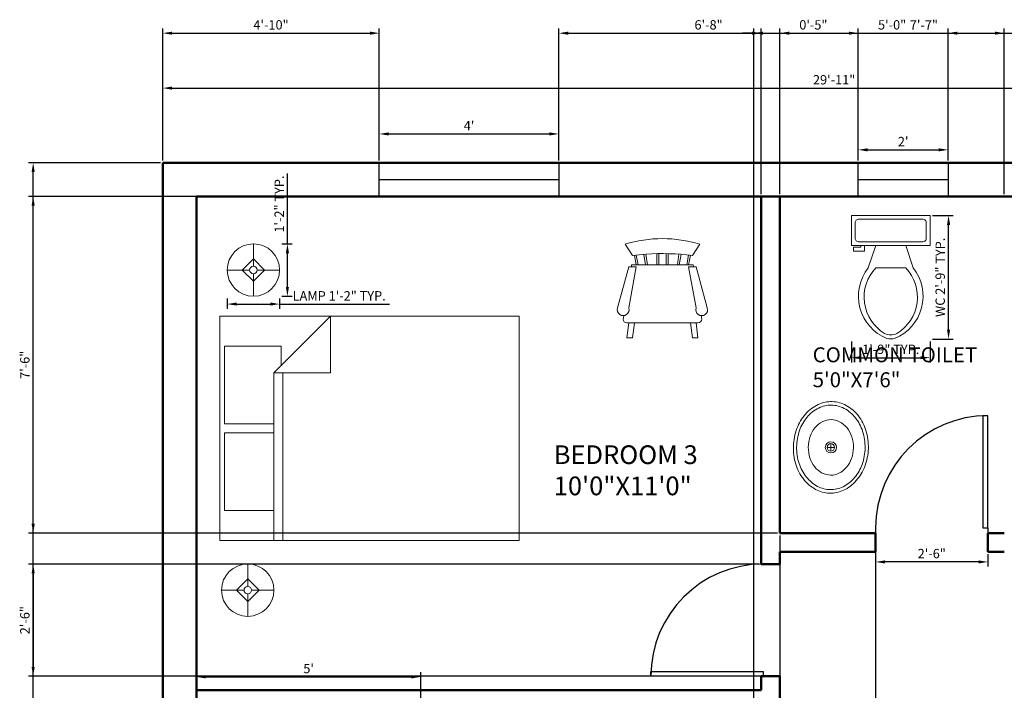
# Model space of a CAD drawing. Units: inches. Extents: x 25547 to 25983, y 30413 to 31159.
# Tile 4 of 5: x 25549 to 25813, y 30978 to 31157. Entities that reach past the tile are written whole.
import ezdxf

# ---------------------------------------------------------------- set-up
doc = ezdxf.new("R2010")
doc.units = ezdxf.units.IN
for name, color, linetype, lineweight in [('A-AREA-IDEN', 11, 'Continuous', 25), ('A-FLOR-FIXT', 6, 'Continuous', 18), ('A-WALL', 7, 'Continuous', 50), ('DIM', 4, 'Continuous', 18), ('DOOR', 3, 'Continuous', 25), ('FURNITURES', 6, 'Continuous', 18), ('WINDOW', 1, 'Continuous', 25)]:
    doc.layers.add(name, color=color, linetype=linetype, lineweight=lineweight)
doc.styles.get("Standard").update_dxf_attribs({"font": 'arial.ttf'})
doc.dimstyles.new('ISO-25', dxfattribs={"dimtxt": 2.5, "dimasz": 2.5, "dimexe": 1.25, "dimexo": 0.625, "dimtad": 1, "dimlunit": 3, "dimtxsty": 'Standard', "dimcen": 2.5, "dimadec": 0, "dimazin": 0, "dimtfac": 1, "dimtmove": 0, "dimatfit": 3, "dimfxl": 1, "dimarcsym": 0})

# ---------------------------------------------------------------- blocks, each defined once
blk = doc.blocks.new('*U5')
for p, q in [((0, 0), (0, -6)), ((40, 0), (40, -6))]:
    blk.add_line(p, q)
blk.add_lwpolyline([(0, 0), (0, 40), (1.75, 40), (1.75, 0)], close=True)
blk.add_arc((0, 0), 40, 0, 90)
blk = doc.blocks.new('*U3')
for p, q in [((0, 0), (0, -6)), ((-40, 0), (-40, -6))]:
    blk.add_line(p, q)
blk.add_lwpolyline([(0, 0), (0, 40), (-1.75, 40), (-1.75, 0)], close=True)
blk.add_arc((0, 0), 40, 90, 180)
blk = doc.blocks.new('Chair - Rocking')
for p, q in [((-8, -4.5), (-10, -1.5)), ((8, -4.5), (10, -1.5)), ((-7.5, -4.5), (-7, -7)), ((-6.5, -7), (-7.02225, -4.43)), ((-4.5, -7), (-4.96674, -4.19951)), ((-4, -7), (-4.40532, -4.16272)), ((-1.5, -4.05012), (-1.5, -7)), ((-1, -7), (-1, -4.05012)), ((1, -7), (1, -4.04655)), ((1.5, -4.05012), (1.5, -7)), ((4, -7), (4.40187, -4.18694)), ((4.5, -7), (4.96761, -4.19437)), ((6.5, -7), (7, -4.4057)), ((7.5, -4.5), (7, -7)), ((-9, -7.5), (-12, -18.49999)), ((-7, -7.5), (-9, -7.5)), ((-9, -18.49999), (-7, -7.5)), ((-8.23428, -6.99939), (-8.3093, -7.47958)), ((-8.23041, -7), (8.23915, -7)), ((7, -7.5), (9, -7.5)), ((9, -18.49999), (7, -7.5)), ((8.31071, -7.48854), (8.23449, -7.00073)), ((9, -7.5), (12, -18.49999)), ((-10.36644, -20.64523), (-10.5, -21.49999)), ((10.5, -21.49999), (10.3575, -20.58798)), ((-9, -22.49999), (-9.5, -26.49999)), ((0, -22.49999), (-9.5, -22.49999)), ((-8, -26.49999), (-7.5, -22.49999)), ((0, -22.49999), (9.5, -22.49999)), ((8, -26.49999), (7.5, -22.49999)), ((9, -22.49999), (9.5, -26.49999)), ((-9.5, -26.49999), (-8, -26.49999)), ((9.5, -26.49999), (8, -26.49999))]:
    blk.add_line(p, q)
for centre, radius, start, end in [((0, -34.08333), 34.08333, 72.93847, 107.0615), ((0, -68.25004), 64.25, 93.92211, 97.15267), ((0, -68.25004), 64.25, 82.84733, 93.92211), ((-10.5, -18.99999), 1.58114, 161.5651, 18.43495), ((10.5, -18.99999), 1.58114, 161.5651, 18.43495), ((-9.5, -21.49999), 1, 180, 270), ((9.5, -21.49999), 1, 270, 0)]:
    blk.add_arc(centre, radius, start, end)
blk = doc.blocks.new('Bed - Queen')
for p, q in [((0, -80.00003), (0, 0)), ((0, 0), (59.99999, 0)), ((59.99999, 0), (59.99999, -80.00003)), ((7.99999, -1.2), (28.79998, -1.2)), ((7.99999, -14.4), (7.99999, -1.2)), ((28.79998, -1.2), (28.79998, -14.4)), ((31.19999, -1.2), (51.99999, -1.2)), ((31.19999, -14.4), (31.19999, -1.2)), ((51.99999, -1.2), (51.99999, -16.4)), ((0, -14.4), (44.8, -14.4)), ((59.99999, -29.6), (44.8, -14.4)), ((44.8, -14.4), (44.8, -29.6)), ((44.8, -16.8), (0, -16.8)), ((51.99999, -16.4), (46.79936, -16.4)), ((44.8, -29.6), (59.99999, -29.6)), ((59.99999, -80.00003), (0, -80.00003))]:
    blk.add_line(p, q)
blk = doc.blocks.new('Lamp - Table')
for p, q in [((0, 7), (0, 1)), ((0, 3), (-3, 0)), ((3, 0), (0, 3)), ((-1, 0), (-7, 0)), ((-3, 0), (0, -3)), ((0, -3), (3, 0)), ((1, 0), (7, 0)), ((0, -1), (0, -7))]:
    blk.add_line(p, q)
for radius in [7, 1]:
    blk.add_circle((0, 0), radius)
blk = doc.blocks.new('Toilet - top')
for p, q in [((9.5, -6), (9.5, -2)), ((-10, -8.5), (-8, -8.5)), ((-10, -9.5), (-10, -8.5)), ((-7, -9.5), (-10, -9.5)), ((-8, -8.5), (-8, -8)), ((-7, -8), (-7, -9.5)), ((-4, -8), (-6, -14)), ((4, -8), (6, -14)), ((4, -14), (-4, -14))]:
    blk.add_line(p, q)
blk.add_lwpolyline([(10.5, -8), (10.5, 0), (-10.5, 0), (-10.5, -8)], close=True)
for points in [[(-9.5, -2), (-9.5, -6)], [(8.5, -1), (-8.5, -1)], [(-8.5, -7), (8.5, -7)]]:
    blk.add_lwpolyline(points)
for centre, radius, start, end in [((-8.62, -1.88), 0.884, 81.8699, 188.1301), ((8.62, -1.88), 0.884, 351.8699, 98.1301), ((-8.62, -6.12), 0.884, 171.8699, 278.1301), ((8.62, -6.12), 0.884, 261.8699, 8.1301), ((3.52, -21.58), 12.17, 141.4691, 247.9714), ((4.2, -21.82), 11.33, 136.3677, 238.9468), ((-3.52, -21.58), 12.17, 292.0284, 38.5307), ((-4.2, -21.82), 11.33, 301.053, 43.6321), ((0, -27.88), 4, 245.7318, 294.2682), ((0, -29), 4, 254.8605, 285.1395)]:
    blk.add_arc(centre, radius, start, end)
blk = doc.blocks.new('Sink - Oval top')
for p, q in [((-1, 0), (1, 0)), ((0, 1), (0, -1))]:
    blk.add_line(p, q)
for points in [[(-12.23, 0.39, 0.117634), (-11.46, -3.36, 0.104469), (-8.88, -6.8, 0.090016), (-5.08, -9.07, 0.08192), (-0.32, -10.02, 0.08192), (4.49, -9.38, 0.090016), (8.42, -7.36, 0.104469), (11.22, -4.09, 0.117634), (12.23, -0.39, 0.117634), (11.46, 3.36, 0.104469), (8.88, 6.8, 0.090016), (5.08, 9.07, 0.08192), (0.32, 10.02, 0.08192), (-4.49, 9.38, 0.090016), (-8.42, 7.36, 0.104469), (-11.22, 4.09, 0.117634)], [(-11.29, 0.16, 0.118622), (-10.52, -3.25, 0.104678), (-8.07, -6.36, 0.089562), (-4.54, -8.37, 0.081185), (-0.13, -9.15, 0.081185), (4.3, -8.49, 0.089562), (7.89, -6.58, 0.104678), (10.42, -3.55, 0.118622), (11.29, -0.16, 0.118622), (10.52, 3.25, 0.104678), (8.07, 6.36, 0.089562), (4.54, 8.37, 0.081185), (0.13, 9.15, 0.081185), (-4.3, 8.49, 0.089562), (-7.89, 6.58, 0.104678), (-10.42, 3.55, 0.118622)], [(-7.42, 0.08, 0.118283), (-6.91, -2.17, 0.104607), (-5.29, -4.21, 0.089718), (-2.97, -5.53, 0.081436), (-0.07, -6.04, 0.081436), (2.84, -5.59, 0.089718), (5.2, -4.33, 0.104607), (6.86, -2.32, 0.118283), (7.42, -0.08, 0.118283), (6.91, 2.17, 0.104607), (5.29, 4.21, 0.089718), (2.97, 5.53, 0.081436), (0.07, 6.04, 0.081436), (-2.84, 5.59, 0.089718), (-5.2, 4.33, 0.104607), (-6.86, 2.32, 0.118283)]]:
    blk.add_lwpolyline(points, format="xyb", close=True)
for radius in [1.5, 1]:
    blk.add_circle((0, 0), radius)
blk = doc.blocks.new('*D22')
at = {"layer": 'Defpoints', "color": 0, "transparency": 16777216}
for p in [(25693.43, 31126.54), (25645.43, 31118.83), (25693.43, 31118.83)]:
    blk.add_point(p, dxfattribs=at)
at = {"layer": 'DIM', "color": 0, "lineweight": -2, "transparency": 16777216}
for p, q in [((25645.43, 31119.45), (25645.43, 31127.79)), ((25647.93, 31126.54), (25690.93, 31126.54)), ((25693.43, 31119.45), (25693.43, 31127.79))]:
    blk.add_line(p, q, dxfattribs=at)
at = {"layer": 'DIM', "color": 0, "transparency": 16777216}
for points in [[(25647.93, 31126.95), (25647.93, 31126.12), (25645.43, 31126.54)], [(25690.93, 31126.95), (25690.93, 31126.12), (25693.43, 31126.54)]]:
    blk.add_solid(points, dxfattribs=at)
at = {"layer": 'DIM', "color": 0, "transparency": 16777216, "insert": (25669.43, 31128.41), "char_height": 2.5, "attachment_point": 5}
blk.add_mtext("4'", dxfattribs=at)
blk = doc.blocks.new('*D23')
at = {"layer": 'Defpoints', "color": 0, "transparency": 16777216}
for p in [(25946.53, 31138.79), (25587.53, 31118.83), (25946.53, 31118.83)]:
    blk.add_point(p, dxfattribs=at)
at = {"layer": 'DIM', "color": 0, "lineweight": -2, "transparency": 16777216}
for p, q in [((25587.53, 31119.45), (25587.53, 31140.04)), ((25946.53, 31119.45), (25946.53, 31140.04)), ((25590.03, 31138.79), (25944.03, 31138.79))]:
    blk.add_line(p, q, dxfattribs=at)
at = {"layer": 'DIM', "color": 0, "transparency": 16777216}
for points in [[(25590.03, 31139.21), (25590.03, 31138.37), (25587.53, 31138.79)], [(25944.03, 31139.21), (25944.03, 31138.37), (25946.53, 31138.79)]]:
    blk.add_solid(points, dxfattribs=at)
at = {"layer": 'DIM', "color": 0, "transparency": 16777216, "insert": (25767.03, 31140.69), "char_height": 2.5, "attachment_point": 5}
blk.add_mtext('29\'-11"', dxfattribs=at)
blk = doc.blocks.new('*D24')
at = {"layer": 'Defpoints', "color": 0, "transparency": 16777216}
for p in [(25778.13, 31014.83), (25808.13, 31014.83), (25778.13, 31012.14)]:
    blk.add_point(p, dxfattribs=at)
at = {"layer": 'DIM', "color": 0, "lineweight": -2, "transparency": 16777216}
for p, q in [((25778.13, 31014.2), (25778.13, 31010.89)), ((25808.13, 31014.2), (25808.13, 31010.89)), ((25805.63, 31012.14), (25780.63, 31012.14))]:
    blk.add_line(p, q, dxfattribs=at)
at = {"layer": 'DIM', "color": 0, "transparency": 16777216}
for points in [[(25780.63, 31012.56), (25780.63, 31011.72), (25778.13, 31012.14)], [(25805.63, 31012.56), (25805.63, 31011.72), (25808.13, 31012.14)]]:
    blk.add_solid(points, dxfattribs=at)
at = {"layer": 'DIM', "color": 0, "transparency": 16777216, "insert": (25793.13, 31014.04), "char_height": 2.5, "attachment_point": 5}
blk.add_mtext('2\'-6"', dxfattribs=at)
blk = doc.blocks.new('*D31')
at = {"layer": 'Defpoints', "color": 0, "transparency": 16777216}
for p in [(25656.53, 30981.43), (25596.53, 30972.83), (25656.53, 30972.83)]:
    blk.add_point(p, dxfattribs=at)
at = {"layer": 'DIM', "color": 0, "lineweight": -2, "transparency": 16777216}
for p, q in [((25596.53, 30973.45), (25596.53, 30982.68)), ((25599.03, 30981.43), (25654.03, 30981.43)), ((25656.53, 30973.45), (25656.53, 30982.68))]:
    blk.add_line(p, q, dxfattribs=at)
at = {"layer": 'DIM', "color": 0, "transparency": 16777216}
for points in [[(25599.03, 30981.85), (25599.03, 30981.01), (25596.53, 30981.43)], [(25654.03, 30981.85), (25654.03, 30981.01), (25656.53, 30981.43)]]:
    blk.add_solid(points, dxfattribs=at)
at = {"layer": 'DIM', "color": 0, "transparency": 16777216, "insert": (25626.53, 30983.32), "char_height": 2.5, "attachment_point": 5}
blk.add_mtext("5'", dxfattribs=at)
blk = doc.blocks.new('*D32')
at = {"layer": 'Defpoints', "color": 0, "transparency": 16777216}
for p in [(25797.49, 31122.29), (25773.49, 31118.83), (25797.49, 31118.83)]:
    blk.add_point(p, dxfattribs=at)
at = {"layer": 'DIM', "color": 0, "lineweight": -2, "transparency": 16777216}
for p, q in [((25773.49, 31119.45), (25773.49, 31123.54)), ((25797.49, 31119.45), (25797.49, 31123.54)), ((25775.99, 31122.29), (25794.99, 31122.29))]:
    blk.add_line(p, q, dxfattribs=at)
at = {"layer": 'DIM', "color": 0, "transparency": 16777216}
for points in [[(25775.99, 31122.7), (25775.99, 31121.87), (25773.49, 31122.29)], [(25794.99, 31122.7), (25794.99, 31121.87), (25797.49, 31122.29)]]:
    blk.add_solid(points, dxfattribs=at)
at = {"layer": 'DIM', "color": 0, "transparency": 16777216, "insert": (25785.49, 31124.17), "char_height": 2.5, "attachment_point": 5}
blk.add_mtext("2'", dxfattribs=at)
blk = doc.blocks.new('WIN-48IN')
blk.add_line((4.5, 48), (4.5, 0))
blk.add_lwpolyline([(0, 48), (9, 48), (9, 0), (0, 0)], close=True)
blk = doc.blocks.new('WIN-24IN')
blk.add_line((0, 4.5), (24, 4.5))
blk.add_lwpolyline([(0, 0), (0, 9), (24, 9), (24, 0)], close=True)
blk = doc.blocks.new('*D38')
at = {"layer": 'Defpoints', "color": 0, "transparency": 16777216}
for p in [(25604.77, 31083.16), (25618.77, 31083.16), (25618.77, 31081.06)]:
    blk.add_point(p, dxfattribs=at)
at = {"layer": 'DIM', "color": 0, "lineweight": -2, "transparency": 16777216}
for p, q in [((25604.77, 31082.54), (25604.77, 31079.81)), ((25607.27, 31081.06), (25616.27, 31081.06)), ((25618.77, 31082.54), (25618.77, 31079.81)), ((25618.77, 31081.06), (25648.12, 31081.06))]:
    blk.add_line(p, q, dxfattribs=at)
at = {"layer": 'DIM', "color": 0, "transparency": 16777216}
for points in [[(25607.27, 31081.48), (25607.27, 31080.65), (25604.77, 31081.06)], [(25616.27, 31081.48), (25616.27, 31080.65), (25618.77, 31081.06)]]:
    blk.add_solid(points, dxfattribs=at)
at = {"layer": 'DIM', "color": 0, "transparency": 16777216, "insert": (25634.7, 31082.94), "char_height": 2.5, "attachment_point": 5}
blk.add_mtext('LAMP 1\'-2" TYP.', dxfattribs=at)
blk = doc.blocks.new('*D39')
at = {"layer": 'Defpoints', "color": 0, "transparency": 16777216}
for p in [(25618.77, 31097.16), (25620.87, 31097.16), (25618.77, 31083.16)]:
    blk.add_point(p, dxfattribs=at)
at = {"layer": 'DIM', "color": 0, "lineweight": -2, "transparency": 16777216}
for p, q in [((25620.87, 31097.16), (25620.87, 31115.92)), ((25619.39, 31097.16), (25622.12, 31097.16)), ((25620.87, 31085.66), (25620.87, 31094.66)), ((25619.39, 31083.16), (25622.12, 31083.16))]:
    blk.add_line(p, q, dxfattribs=at)
at = {"layer": 'DIM', "color": 0, "transparency": 16777216}
for points in [[(25620.45, 31094.66), (25621.28, 31094.66), (25620.87, 31097.16)], [(25620.45, 31085.66), (25621.28, 31085.66), (25620.87, 31083.16)]]:
    blk.add_solid(points, dxfattribs=at)
at = {"layer": 'DIM', "color": 0, "transparency": 16777216, "insert": (25618.99, 31107.79), "char_height": 2.5, "attachment_point": 5, "rotation": 90}
blk.add_mtext('1\'-2" TYP.', dxfattribs=at)
blk = doc.blocks.new('*D50')
at = {"layer": 'Defpoints', "color": 0, "transparency": 16777216}
for p in [(25792.67, 31104.74), (25797.62, 31104.74), (25792.67, 31071.69)]:
    blk.add_point(p, dxfattribs=at)
at = {"layer": 'DIM', "color": 0, "lineweight": -2, "transparency": 16777216}
for p, q in [((25793.29, 31104.74), (25798.87, 31104.74)), ((25797.62, 31074.19), (25797.62, 31102.24)), ((25793.29, 31071.69), (25798.87, 31071.69))]:
    blk.add_line(p, q, dxfattribs=at)
at = {"layer": 'DIM', "color": 0, "transparency": 16777216}
for points in [[(25797.21, 31102.24), (25798.04, 31102.24), (25797.62, 31104.74)], [(25797.21, 31074.19), (25798.04, 31074.19), (25797.62, 31071.69)]]:
    blk.add_solid(points, dxfattribs=at)
at = {"layer": 'DIM', "color": 0, "transparency": 16777216, "insert": (25795.71, 31088.21), "char_height": 2.5, "attachment_point": 5, "rotation": 90}
blk.add_mtext('WC 2\'-9" TYP.', dxfattribs=at)
blk = doc.blocks.new('*D51')
at = {"layer": 'Defpoints', "color": 0, "transparency": 16777216}
for p in [(25771.67, 31071.69), (25792.67, 31071.69), (25792.67, 31066.73)]:
    blk.add_point(p, dxfattribs=at)
at = {"layer": 'DIM', "color": 0, "lineweight": -2, "transparency": 16777216}
for p, q in [((25771.67, 31071.07), (25771.67, 31065.48)), ((25792.67, 31071.07), (25792.67, 31065.48)), ((25774.17, 31066.73), (25790.17, 31066.73))]:
    blk.add_line(p, q, dxfattribs=at)
at = {"layer": 'DIM', "color": 0, "transparency": 16777216}
for points in [[(25774.17, 31067.15), (25774.17, 31066.32), (25771.67, 31066.73)], [(25790.17, 31067.15), (25790.17, 31066.32), (25792.67, 31066.73)]]:
    blk.add_solid(points, dxfattribs=at)
at = {"layer": 'DIM', "color": 0, "transparency": 16777216, "insert": (25782.17, 31068.64), "char_height": 2.5, "attachment_point": 5}
blk.add_mtext('1\'-9" TYP.', dxfattribs=at)
blk = doc.blocks.new('*D68')
at = {"layer": 'Defpoints', "color": 0, "transparency": 16777216}
for p in [(25552.89, 31118.83), (25587.53, 31118.83), (25587.53, 30449.83)]:
    blk.add_point(p, dxfattribs=at)
at = {"layer": 'DIM', "color": 0, "lineweight": -2, "transparency": 16777216}
for p, q in [((25586.9, 31118.83), (25551.64, 31118.83)), ((25552.89, 30452.33), (25552.89, 31116.33)), ((25586.9, 30449.83), (25551.64, 30449.83))]:
    blk.add_line(p, q, dxfattribs=at)
at = {"layer": 'DIM', "color": 0, "transparency": 16777216}
for points in [[(25552.47, 31116.33), (25553.31, 31116.33), (25552.89, 31118.83)], [(25552.47, 30452.33), (25553.31, 30452.33), (25552.89, 30449.83)]]:
    blk.add_solid(points, dxfattribs=at)
at = {"layer": 'DIM', "color": 0, "transparency": 16777216, "insert": (25550.99, 30784.33), "char_height": 2.5, "attachment_point": 5, "rotation": 90}
blk.add_mtext('55\'-9"', dxfattribs=at)
blk = doc.blocks.new('*D73')
at = {"layer": 'Defpoints', "color": 0, "transparency": 16777216}
for p in [(25645.43, 31153.47), (25587.53, 31118.83), (25645.43, 31118.83)]:
    blk.add_point(p, dxfattribs=at)
at = {"layer": 'DIM', "color": 0, "lineweight": -2, "transparency": 16777216}
for p, q in [((25587.53, 31119.45), (25587.53, 31154.72)), ((25590.03, 31153.47), (25642.93, 31153.47)), ((25645.43, 31119.45), (25645.43, 31154.72))]:
    blk.add_line(p, q, dxfattribs=at)
at = {"layer": 'DIM', "color": 0, "transparency": 16777216}
for points in [[(25590.03, 31153.88), (25590.03, 31153.05), (25587.53, 31153.47)], [(25642.93, 31153.88), (25642.93, 31153.05), (25645.43, 31153.47)]]:
    blk.add_solid(points, dxfattribs=at)
at = {"layer": 'DIM', "color": 0, "transparency": 16777216, "insert": (25616.48, 31155.37), "char_height": 2.5, "attachment_point": 5}
blk.add_mtext('4\'-10"', dxfattribs=at)
blk = doc.blocks.new('*D74')
at = {"layer": 'Defpoints', "color": 0, "transparency": 16777216}
for p in [(25773.49, 31153.47), (25693.43, 31118.83), (25773.49, 31118.83)]:
    blk.add_point(p, dxfattribs=at)
at = {"layer": 'DIM', "color": 0, "lineweight": -2, "transparency": 16777216}
for p, q in [((25693.43, 31119.45), (25693.43, 31154.72)), ((25695.93, 31153.47), (25770.99, 31153.47)), ((25773.49, 31119.45), (25773.49, 31154.72))]:
    blk.add_line(p, q, dxfattribs=at)
at = {"layer": 'DIM', "color": 0, "transparency": 16777216}
for points in [[(25695.93, 31153.88), (25695.93, 31153.05), (25693.43, 31153.47)], [(25770.99, 31153.88), (25770.99, 31153.05), (25773.49, 31153.47)]]:
    blk.add_solid(points, dxfattribs=at)
at = {"layer": 'DIM', "color": 0, "transparency": 16777216, "insert": (25733.46, 31155.37), "char_height": 2.5, "attachment_point": 5}
blk.add_mtext('6\'-8"', dxfattribs=at)
blk = doc.blocks.new('*D75')
at = {"layer": 'Defpoints', "color": 0, "transparency": 16777216}
for p in [(25856.38, 31153.47), (25797.49, 31118.83), (25856.38, 31118.83)]:
    blk.add_point(p, dxfattribs=at)
at = {"layer": 'DIM', "color": 0, "lineweight": -2, "transparency": 16777216}
for p, q in [((25797.49, 31119.45), (25797.49, 31154.72)), ((25799.99, 31153.47), (25853.88, 31153.47)), ((25856.38, 31119.45), (25856.38, 31154.72))]:
    blk.add_line(p, q, dxfattribs=at)
at = {"layer": 'DIM', "color": 0, "transparency": 16777216}
for points in [[(25799.99, 31153.88), (25799.99, 31153.05), (25797.49, 31153.47)], [(25853.88, 31153.88), (25853.88, 31153.05), (25856.38, 31153.47)]]:
    blk.add_solid(points, dxfattribs=at)
at = {"layer": 'DIM', "color": 0, "transparency": 16777216, "insert": (25826.93, 31155.35), "char_height": 2.5, "attachment_point": 5}
blk.add_mtext('4\'-11"', dxfattribs=at)
blk = doc.blocks.new('*D78')
at = {"layer": 'Defpoints', "color": 0, "transparency": 16777216}
for p in [(25752.53, 31153.47), (25747.53, 31109.83), (25752.53, 31109.83)]:
    blk.add_point(p, dxfattribs=at)
at = {"layer": 'DIM', "color": 0, "lineweight": -2, "transparency": 16777216}
for p, q in [((25745.03, 31153.47), (25742.53, 31153.47)), ((25747.53, 31110.45), (25747.53, 31154.72)), ((25747.53, 31153.47), (25752.53, 31153.47)), ((25752.53, 31110.45), (25752.53, 31154.72)), ((25755.03, 31153.47), (25765.42, 31153.47))]:
    blk.add_line(p, q, dxfattribs=at)
at = {"layer": 'DIM', "color": 0, "transparency": 16777216}
for points in [[(25745.03, 31153.88), (25745.03, 31153.05), (25747.53, 31153.47)], [(25755.03, 31153.88), (25755.03, 31153.05), (25752.53, 31153.47)]]:
    blk.add_solid(points, dxfattribs=at)
at = {"layer": 'DIM', "color": 0, "transparency": 16777216, "insert": (25761.48, 31155.37), "char_height": 2.5, "attachment_point": 5}
blk.add_mtext('0\'-5"', dxfattribs=at)
blk = doc.blocks.new('*D79')
at = {"layer": 'Defpoints', "color": 0, "transparency": 16777216}
for p in [(25812.53, 31153.47), (25752.53, 31109.83), (25812.53, 31109.83)]:
    blk.add_point(p, dxfattribs=at)
at = {"layer": 'DIM', "color": 0, "lineweight": -2, "transparency": 16777216}
for p, q in [((25752.53, 31110.45), (25752.53, 31154.72)), ((25755.03, 31153.47), (25810.03, 31153.47)), ((25812.53, 31110.45), (25812.53, 31154.72))]:
    blk.add_line(p, q, dxfattribs=at)
at = {"layer": 'DIM', "color": 0, "transparency": 16777216}
for points in [[(25755.03, 31153.88), (25755.03, 31153.05), (25752.53, 31153.47)], [(25810.03, 31153.88), (25810.03, 31153.05), (25812.53, 31153.47)]]:
    blk.add_solid(points, dxfattribs=at)
at = {"layer": 'DIM', "color": 0, "transparency": 16777216, "insert": (25782.53, 31155.37), "char_height": 2.5, "attachment_point": 5}
blk.add_mtext('5\'-0"', dxfattribs=at)
blk = doc.blocks.new('*D97')
at = {"layer": 'Defpoints', "color": 0, "transparency": 16777216}
for p in [(25552.89, 31109.83), (25752.53, 31109.83), (25752.53, 31019.83)]:
    blk.add_point(p, dxfattribs=at)
at = {"layer": 'DIM', "color": 0, "lineweight": -2, "transparency": 16777216}
for p, q in [((25751.9, 31109.83), (25551.64, 31109.83)), ((25552.89, 31022.33), (25552.89, 31107.33)), ((25751.9, 31019.83), (25551.64, 31019.83))]:
    blk.add_line(p, q, dxfattribs=at)
at = {"layer": 'DIM', "color": 0, "transparency": 16777216}
for points in [[(25552.47, 31107.33), (25553.31, 31107.33), (25552.89, 31109.83)], [(25552.47, 31022.33), (25553.31, 31022.33), (25552.89, 31019.83)]]:
    blk.add_solid(points, dxfattribs=at)
at = {"layer": 'DIM', "color": 0, "transparency": 16777216, "insert": (25550.99, 31064.83), "char_height": 2.5, "attachment_point": 5, "rotation": 90}
blk.add_mtext('7\'-6"', dxfattribs=at)
blk = doc.blocks.new('*D99')
at = {"layer": 'Defpoints', "color": 0, "transparency": 16777216}
for p in [(25836.53, 31153.47), (25745.53, 30799.83), (25836.53, 30794.83)]:
    blk.add_point(p, dxfattribs=at)
at = {"layer": 'DIM', "color": 0, "lineweight": -2, "transparency": 16777216}
for p, q in [((25745.53, 30800.45), (25745.53, 31154.72)), ((25748.03, 31153.47), (25834.03, 31153.47)), ((25836.53, 30795.45), (25836.53, 31154.72))]:
    blk.add_line(p, q, dxfattribs=at)
at = {"layer": 'DIM', "color": 0, "transparency": 16777216}
for points in [[(25748.03, 31153.88), (25748.03, 31153.05), (25745.53, 31153.47)], [(25834.03, 31153.88), (25834.03, 31153.05), (25836.53, 31153.47)]]:
    blk.add_solid(points, dxfattribs=at)
at = {"layer": 'DIM', "color": 0, "transparency": 16777216, "insert": (25791.03, 31155.34), "char_height": 2.5, "attachment_point": 5}
blk.add_mtext('7\'-7"', dxfattribs=at)
blk = doc.blocks.new('*D100')
at = {"layer": 'Defpoints', "color": 0, "transparency": 16777216}
for p in [(25747.53, 31011.57), (25552.89, 30981.57), (25747.53, 30981.57)]:
    blk.add_point(p, dxfattribs=at)
at = {"layer": 'DIM', "color": 0, "lineweight": -2, "transparency": 16777216}
for p, q in [((25746.9, 31011.57), (25551.64, 31011.57)), ((25552.89, 31009.07), (25552.89, 30984.07)), ((25746.9, 30981.57), (25551.64, 30981.57))]:
    blk.add_line(p, q, dxfattribs=at)
at = {"layer": 'DIM', "color": 0, "transparency": 16777216}
for points in [[(25552.47, 31009.07), (25553.31, 31009.07), (25552.89, 31011.57)], [(25552.47, 30984.07), (25553.31, 30984.07), (25552.89, 30981.57)]]:
    blk.add_solid(points, dxfattribs=at)
at = {"layer": 'DIM', "color": 0, "transparency": 16777216, "insert": (25550.99, 30996.57), "char_height": 2.5, "attachment_point": 5, "rotation": 90}
blk.add_mtext('2\'-6"', dxfattribs=at)
blk = doc.blocks.new('*D103')
at = {"layer": 'Defpoints', "color": 0, "transparency": 16777216}
for p in [(25752.53, 31019.83), (25778.13, 31019.83), (25778.13, 30415.19)]:
    blk.add_point(p, dxfattribs=at)
at = {"layer": 'DIM', "color": 0, "lineweight": -2, "transparency": 16777216}
for p, q in [((25752.53, 31019.2), (25752.53, 30413.94)), ((25778.13, 31019.2), (25778.13, 30413.94)), ((25755.03, 30415.19), (25775.63, 30415.19))]:
    blk.add_line(p, q, dxfattribs=at)
at = {"layer": 'DIM', "color": 0, "transparency": 16777216}
for points in [[(25755.03, 30415.61), (25755.03, 30414.77), (25752.53, 30415.19)], [(25775.63, 30415.61), (25775.63, 30414.77), (25778.13, 30415.19)]]:
    blk.add_solid(points, dxfattribs=at)
at = {"layer": 'DIM', "color": 0, "transparency": 16777216, "insert": (25765.33, 30417.11), "char_height": 2.5, "attachment_point": 5}
blk.add_mtext('2\'-1 1/2"', dxfattribs=at)

msp = doc.modelspace()

# ---------------------------------------------------------------- linework, layer by layer
at = {"layer": 'A-WALL'}
for p, q in [((25587.528, 31118.828), (25946.528, 31118.828)), ((25587.528, 30852.828), (25587.528, 31118.828)), ((25596.528, 31109.828), (25937.528, 31109.828)), ((25596.528, 30650.828), (25596.528, 31109.828)), ((25747.528, 31011.569), (25747.528, 31109.828)), ((25752.528, 31019.828), (25752.528, 31109.828)), ((25752.528, 31019.828), (25778.126, 31019.828)), ((25808.126, 31019.828), (25812.528, 31019.828)), ((25752.528, 31014.828), (25778.126, 31014.828)), ((25752.528, 31011.569), (25752.528, 31014.828)), ((25808.126, 31014.828), (25812.528, 31014.828)), ((25747.528, 30977.828), (25747.528, 30981.569)), ((25752.528, 30972.828), (25752.528, 30981.569)), ((25596.528, 30977.828), (25747.528, 30977.828))]:
    msp.add_line(p, q, dxfattribs=at)
for points in [[(25778.126, 31014.828), (25778.126, 31019.828)], [(25808.126, 31019.828), (25808.126, 31014.828)], [(25747.528, 31011.569), (25752.528, 31011.569)], [(25752.528, 30981.569), (25747.528, 30981.569)]]:
    msp.add_lwpolyline(points, dxfattribs=at)

# ---------------------------------------------------------------- block references
at = {"layer": 'A-FLOR-FIXT'}
msp.add_blockref('Toilet - top', (25782.167, 31104.737), dxfattribs=at)
at = {"layer": 'A-FLOR-FIXT', "rotation": 90}
msp.add_blockref('Sink - Oval top', (25766.159, 31042.759), dxfattribs=at)
at = {"layer": 'DOOR', "xscale": 0.75, "yscale": 0.75, "zscale": 0.75}
msp.add_blockref('*U3', (25808.126, 31021.233), dxfattribs=at)
at = {"layer": 'DOOR', "xscale": 0.75, "yscale": 0.75, "zscale": 0.75, "rotation": 90}
msp.add_blockref('*U5', (25748.028, 30981.569), dxfattribs=at)
at = {"layer": 'FURNITURES'}
for name, p in [('Lamp - Table', (25611.766, 31090.163)), ('Chair - Rocking', (25721.128, 31098.553)), ('Lamp - Table', (25610.266, 31004.591))]:
    msp.add_blockref(name, p, dxfattribs=at)
at = {"layer": 'FURNITURES', "rotation": 90}
msp.add_blockref('Bed - Queen', (25602.805, 31017.85), dxfattribs=at)
at = {"layer": 'WINDOW', "rotation": 89.99999999998533}
msp.add_blockref('WIN-48IN', (25693.425, 31109.828), dxfattribs=at)
at = {"layer": 'WINDOW'}
msp.add_blockref('WIN-24IN', (25773.486, 31109.828), dxfattribs=at)

# ---------------------------------------------------------------- texts
at = {"layer": 'A-AREA-IDEN', "attachment_point": 1}
for s, insert, char_height in [('{\\fArial|b1|i1|c0|p34;COMMON TOILET\\P5\'0"X7\'6"}', (25761.294, 31069.502), 4), ('{\\fArial|b1|i1|c0|p34;BEDROOM 3\\P10\'0"X11\'0"}', (25692.065, 31043.3), 5)]:
    msp.add_mtext_dynamic_manual_height_columns(s, width=113.82935, gutter_width=18.048, heights=[0], dxfattribs=dict(at, insert=insert, char_height=char_height))

# ---------------------------------------------------------------- dimensions: what is measured, and where the dimension line sits
at = {"layer": 'DIM'}
for base, p1, p2, override, picture, middle in [((25645.425, 31153.465), (25587.528, 31118.828), (25645.425, 31118.828), {"dimdec": 1, "dimlfac": 1, "dimrnd": 0, "dimzin": 1, "dimdsep": 46, "dimlunit": 4, "dimfrac": 2}, '*D73', (25616.477, 31155.367)), ((25773.486, 31153.465), (25693.425, 31118.828), (25773.486, 31118.828), {"dimdec": 1, "dimlfac": 1, "dimrnd": 0, "dimzin": 1, "dimdsep": 46, "dimlunit": 4, "dimfrac": 2}, '*D74', (25733.456, 31155.367)), ((25752.528, 31153.465), (25747.528, 31109.828), (25752.528, 31109.828), {"dimdec": 1, "dimlfac": 1, "dimrnd": 0, "dimzin": 1, "dimdsep": 46, "dimlunit": 4, "dimfrac": 2}, '*D78', (25761.476, 31155.367)), ((25836.528, 31153.465), (25745.528, 30799.828), (25836.528, 30794.828), {"dimdec": 1, "dimlfac": 1, "dimrnd": 0, "dimzin": 1, "dimdsep": 46, "dimlunit": 4, "dimfrac": 2}, '*D99', (25791.028, 31155.34)), ((25812.528, 31153.465), (25752.528, 31109.828), (25812.528, 31109.828), {"dimdec": 1, "dimlfac": 1, "dimrnd": 0, "dimzin": 1, "dimdsep": 46, "dimlunit": 4, "dimfrac": 2}, '*D79', (25782.528, 31155.367)), ((25856.375, 31153.465), (25797.486, 31118.828), (25856.375, 31118.828), {"dimdec": 1, "dimlfac": 1, "dimrnd": 0, "dimzin": 1, "dimdsep": 46, "dimlunit": 4, "dimfrac": 2}, '*D75', (25826.931, 31155.346)), ((25946.528, 31138.789), (25587.528, 31118.828), (25946.528, 31118.828), {"dimclrd": 0, "dimclre": 0, "dimclrt": 0}, '*D23', (25767.028, 31140.69)), ((25693.425, 31126.537), (25645.425, 31118.828), (25693.425, 31118.828), {"dimclrd": 0, "dimclre": 0, "dimclrt": 0}, '*D22', (25669.425, 31128.412)), ((25797.486, 31122.285), (25773.486, 31118.828), (25797.486, 31118.828), {"dimclrd": 0, "dimclre": 0, "dimclrt": 0}, '*D32', (25785.486, 31124.165)), ((25778.126, 30415.19), (25752.528, 31019.828), (25778.126, 31019.828), {"dimdec": 1, "dimlfac": 1, "dimrnd": 0, "dimzin": 1, "dimdsep": 46, "dimlunit": 4, "dimfrac": 2}, '*D103', (25765.327, 30417.108)), ((25778.126, 31012.141), (25808.126, 31014.828), (25778.126, 31014.828), {"dimclrd": 0, "dimclre": 0, "dimclrt": 0}, '*D24', (25793.126, 31014.043)), ((25656.528, 30981.429), (25596.528, 30972.828), (25656.528, 30972.828), {"dimclrd": 0, "dimclre": 0, "dimclrt": 0}, '*D31', (25626.528, 30983.325))]:
    dim = msp.add_linear_dim(base=base, p1=p1, p2=p2, dimstyle='ISO-25', override=override, dxfattribs=at)
    dim.commit()
    dim.dimension.update_dxf_attribs({"geometry": picture, "text_midpoint": middle})
for base, p1, p2, picture, middle in [((25552.891, 31118.828), (25587.528, 30449.828), (25587.528, 31118.828), '*D68', (25550.989, 30784.328)), ((25552.891, 31109.828), (25752.528, 31019.828), (25752.528, 31109.828), '*D97', (25550.989, 31064.828)), ((25552.891, 30981.569), (25747.528, 31011.569), (25747.528, 30981.569), '*D100', (25550.989, 30996.569))]:
    dim = msp.add_linear_dim(base=base, p1=p1, p2=p2, angle=90, dimstyle='ISO-25', override={"dimdec": 1, "dimlfac": 1, "dimrnd": 0, "dimzin": 1, "dimdsep": 46, "dimlunit": 4, "dimfrac": 2}, dxfattribs=at)
    dim.commit()
    dim.dimension.update_dxf_attribs({"geometry": picture, "text_midpoint": middle})
for base, p1, p2, text, picture, middle in [((25620.866, 31097.163), (25618.766, 31083.163), (25618.766, 31097.163), '<> TYP.', '*D39', (25618.985, 31107.789)), ((25797.624, 31104.737), (25792.667, 31071.691), (25792.667, 31104.737), 'WC <> TYP.', '*D50', (25795.706, 31088.214))]:
    dim = msp.add_linear_dim(base=base, p1=p1, p2=p2, angle=90, text=text, dimstyle='ISO-25', override={"dimdec": 1, "dimlfac": 1, "dimrnd": 0, "dimzin": 1, "dimdsep": 46, "dimlunit": 4, "dimfrac": 2}, dxfattribs=at)
    dim.commit()
    dim.dimension.update_dxf_attribs({"geometry": picture, "text_midpoint": middle})
for base, p1, p2, text, picture, middle in [((25618.766, 31081.063), (25604.766, 31083.163), (25618.766, 31083.163), 'LAMP <> TYP.', '*D38', (25634.695, 31082.944)), ((25792.667, 31066.734), (25771.667, 31071.691), (25792.667, 31071.691), '<> TYP.', '*D51', (25782.167, 31068.635))]:
    dim = msp.add_linear_dim(base=base, p1=p1, p2=p2, text=text, dimstyle='ISO-25', override={"dimdec": 1, "dimlfac": 1, "dimrnd": 0, "dimzin": 1, "dimdsep": 46, "dimlunit": 4, "dimfrac": 2}, dxfattribs=at)
    dim.commit()
    dim.dimension.update_dxf_attribs({"geometry": picture, "text_midpoint": middle})

doc.saveas('drawing.dxf')
